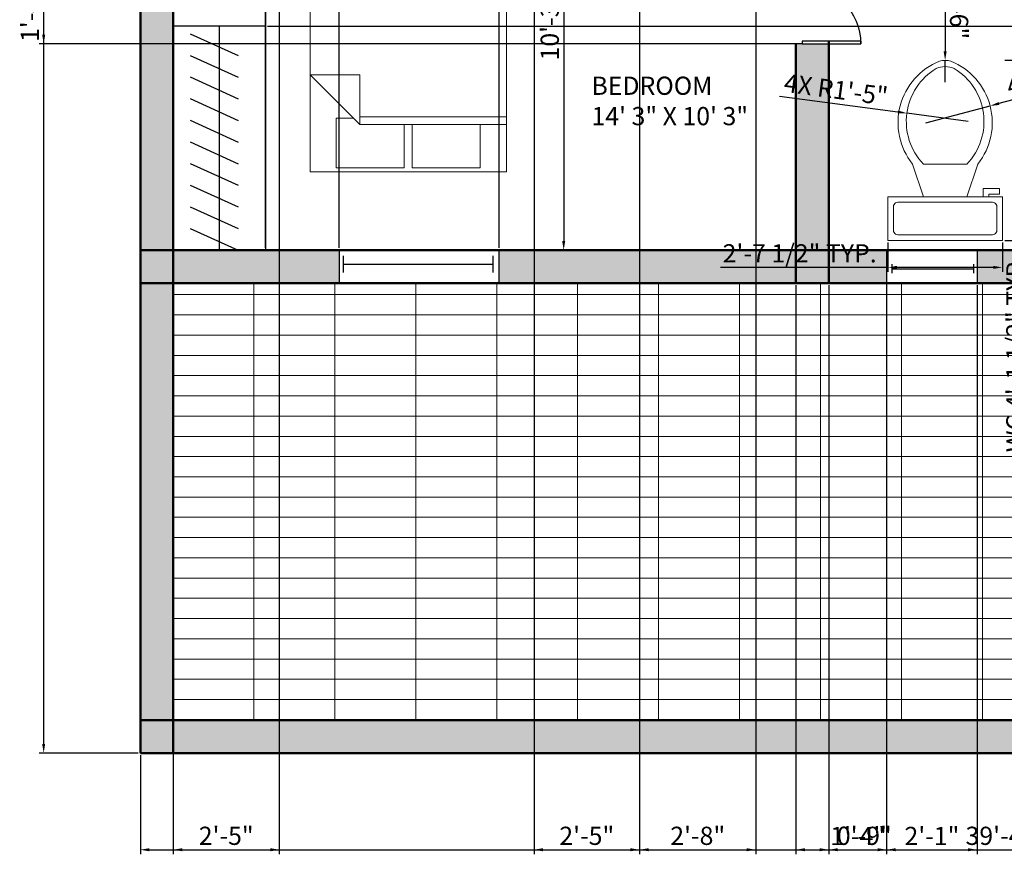
# Model space of a CAD drawing. Units: millimetres. Extents: x 2976 to 3516, y 849 to 1445.
# Tile 1 of 7: x 2981 to 3251, y 852 to 1081. Entities that reach past the tile are written whole.
import ezdxf

# ---------------------------------------------------------------- set-up
doc = ezdxf.new("R2010")
doc.units = ezdxf.units.MM
for name, color, linetype, lineweight in [('A-AREA-IDEN', 150, 'Continuous', 25), ('A-FLOR-CASE', 130, 'Continuous', 25), ('A-FLOR-FIXT', 130, 'Continuous', 18), ('A-FLOR-PATT', 3, 'Continuous', 13), ('A-WALL-PATT', 3, 'Continuous', 13), ('dimensions', 50, 'Continuous', 18), ('doors', 190, 'Continuous', 25), ('furniture', 130, 'Continuous', 18), ('walls', 80, 'Continuous', 50), ('windows', 10, 'Continuous', 25)]:
    doc.layers.add(name, color=color, linetype=linetype, lineweight=lineweight)
doc.styles.get("Standard").update_dxf_attribs({"font": 'arial.ttf'})
doc.dimstyles.new('ISO-25', dxfattribs={"dimtxt": 5, "dimasz": 2.5, "dimexe": 1.25, "dimexo": 0.625, "dimtad": 1, "dimdec": 0, "dimlunit": 3, "dimtxsty": 'Standard', "dimcen": 2.5, "dimadec": 0, "dimazin": 0, "dimtfac": 1, "dimtdec": 0, "dimtmove": 0, "dimatfit": 3, "dimfxl": 1, "dimarcsym": 0})

# ---------------------------------------------------------------- blocks, each defined once
blk = doc.blocks.new('*U2')
for p, q in [((0, 0), (0, -6)), ((40, 0), (40, -6))]:
    blk.add_line(p, q)
blk.add_lwpolyline([(0, 0), (0, 40), (1.75, 40), (1.75, 0)], close=True)
blk.add_arc((0, 0), 40, 0, 90)
blk = doc.blocks.new('*U4')
for p, q in [((0, 4), (0, 0)), ((36, 4), (36, 0)), ((0, 2), (36, 2))]:
    blk.add_line(p, q)
blk = doc.blocks.new('*U5')
for p, q in [((0, 4), (0, 0)), ((0, 2), (36, 2)), ((36, 4), (36, 0))]:
    blk.add_line(p, q)
blk = doc.blocks.new('Bed - Queen')
for p, q in [((0, -80.00003), (0, 0)), ((0, 0), (59.99999, 0)), ((59.99999, 0), (59.99999, -80.00003)), ((7.99999, -1.2), (28.79998, -1.2)), ((7.99999, -14.4), (7.99999, -1.2)), ((28.79998, -1.2), (28.79998, -14.4)), ((31.19999, -1.2), (51.99999, -1.2)), ((31.19999, -14.4), (31.19999, -1.2)), ((51.99999, -1.2), (51.99999, -16.4)), ((0, -14.4), (44.8, -14.4)), ((59.99999, -29.6), (44.8, -14.4)), ((44.8, -14.4), (44.8, -29.6)), ((44.8, -16.8), (0, -16.8)), ((51.99999, -16.4), (46.79936, -16.4)), ((44.8, -29.6), (59.99999, -29.6)), ((59.99999, -80.00003), (0, -80.00003))]:
    blk.add_line(p, q)
blk = doc.blocks.new('Toilet - top')
for p, q in [((9.5, -6), (9.5, -2)), ((-10, -8.5), (-8, -8.5)), ((-10, -9.5), (-10, -8.5)), ((-8, -8.5), (-8, -8)), ((-7, -8), (-7, -9.5)), ((-4, -8), (-6, -14)), ((4, -8), (6, -14)), ((-7, -9.5), (-10, -9.5)), ((4, -14), (-4, -14))]:
    blk.add_line(p, q)
blk.add_lwpolyline([(10.5, -8), (10.5, 0), (-10.5, 0), (-10.5, -8)], close=True)
for points in [[(8.5, -1), (-8.5, -1)], [(-9.5, -2), (-9.5, -6)], [(-8.5, -7), (8.5, -7)]]:
    blk.add_lwpolyline(points)
for centre, radius, start, end in [((-8.62, -1.88), 0.884, 81.8699, 188.1301), ((8.62, -1.88), 0.884, 351.8699, 98.1301), ((-8.62, -6.12), 0.884, 171.8699, 278.1301), ((8.62, -6.12), 0.884, 261.8699, 8.1301), ((3.52, -21.58), 12.17, 141.4691, 247.9714), ((4.2, -21.82), 11.33, 136.3677, 238.9468), ((-3.52, -21.58), 12.17, 292.0284, 38.5307), ((-4.2, -21.82), 11.33, 301.053, 43.6321), ((0, -27.88), 4, 245.7318, 294.2682), ((0, -29), 4, 254.8605, 285.1395)]:
    blk.add_arc(centre, radius, start, end)
blk = doc.blocks.new('*D16')
at = {"layer": 'Defpoints', "color": 0, "transparency": 16777216}
for p in [(3129.91, 1140.88), (3129.91, 1017.88), (3129.91, 1017.88)]:
    blk.add_point(p, dxfattribs=at)
at = {"layer": 'dimensions', "color": 0, "lineweight": -2, "transparency": 16777216}
for p, q in [((3130.53, 1140.88), (3131.16, 1140.88)), ((3129.91, 1138.38), (3129.91, 1020.38)), ((3130.53, 1017.88), (3131.16, 1017.88))]:
    blk.add_line(p, q, dxfattribs=at)
at = {"layer": 'dimensions', "color": 0, "transparency": 16777216}
for points in [[(3129.49, 1138.38), (3130.32, 1138.38), (3129.91, 1140.88)], [(3129.49, 1020.38), (3130.32, 1020.38), (3129.91, 1017.88)]]:
    blk.add_solid(points, dxfattribs=at)
at = {"layer": 'dimensions', "color": 0, "transparency": 16777216, "insert": (3126.73, 1079.38), "char_height": 5, "attachment_point": 5, "rotation": 90}
blk.add_mtext('10\'-3"', dxfattribs=at)
blk = doc.blocks.new('*D32')
at = {"layer": 'Defpoints', "color": 0, "transparency": 16777216}
for p in [(3250.35, 1070.03), (3250.35, 1020.59), (3257.77, 1020.59)]:
    blk.add_point(p, dxfattribs=at)
at = {"layer": 'dimensions', "color": 0, "lineweight": -2, "transparency": 16777216}
for p, q in [((3250.98, 1070.03), (3259.02, 1070.03)), ((3257.77, 1067.53), (3257.77, 1023.09)), ((3250.98, 1020.59), (3259.02, 1020.59)), ((3257.77, 1020.59), (3257.77, 960.93))]:
    blk.add_line(p, q, dxfattribs=at)
at = {"layer": 'dimensions', "color": 0, "transparency": 16777216}
for points in [[(3257.35, 1067.53), (3258.18, 1067.53), (3257.77, 1070.03)], [(3257.35, 1023.09), (3258.18, 1023.09), (3257.77, 1020.59)]]:
    blk.add_solid(points, dxfattribs=at)
at = {"layer": 'dimensions', "color": 0, "transparency": 16777216, "insert": (3254.56, 989.51), "char_height": 5, "attachment_point": 5, "rotation": 90}
blk.add_mtext('WC 4\'-1 1/2" TYP.', dxfattribs=at)
blk = doc.blocks.new('*D33')
at = {"layer": 'Defpoints', "color": 0, "transparency": 16777216}
for p in [(3218.93, 1020.59), (3250.35, 1020.59), (3218.93, 1013.17)]:
    blk.add_point(p, dxfattribs=at)
at = {"layer": 'dimensions', "color": 0, "lineweight": -2, "transparency": 16777216}
for p, q in [((3218.93, 1019.97), (3218.93, 1011.92)), ((3250.35, 1019.97), (3250.35, 1011.92)), ((3218.93, 1013.17), (3172.97, 1013.17)), ((3247.85, 1013.17), (3221.43, 1013.17))]:
    blk.add_line(p, q, dxfattribs=at)
at = {"layer": 'dimensions', "color": 0, "transparency": 16777216}
for points in [[(3221.43, 1013.59), (3221.43, 1012.76), (3218.93, 1013.17)], [(3247.85, 1013.59), (3247.85, 1012.76), (3250.35, 1013.17)]]:
    blk.add_solid(points, dxfattribs=at)
at = {"layer": 'dimensions', "color": 0, "transparency": 16777216, "insert": (3194.7, 1016.38), "char_height": 5, "attachment_point": 5}
blk.add_mtext('2\'-7 1/2" TYP.', dxfattribs=at)
blk = doc.blocks.new('*D38')
at = {"layer": 'Defpoints', "color": 0, "transparency": 16777216}
for p in [(3013.67, 879.88), (3485.67, 879.88), (3485.67, 853.34)]:
    blk.add_point(p, dxfattribs=at)
at = {"layer": 'dimensions', "color": 0, "lineweight": -2, "transparency": 16777216}
for p, q in [((3013.67, 879.26), (3013.67, 852.09)), ((3485.67, 879.26), (3485.67, 852.09)), ((3016.17, 853.34), (3483.17, 853.34))]:
    blk.add_line(p, q, dxfattribs=at)
at = {"layer": 'dimensions', "color": 0, "transparency": 16777216}
for points in [[(3016.17, 853.76), (3016.17, 852.92), (3013.67, 853.34)], [(3483.17, 853.76), (3483.17, 852.92), (3485.67, 853.34)]]:
    blk.add_solid(points, dxfattribs=at)
at = {"layer": 'dimensions', "color": 0, "transparency": 16777216, "insert": (3249.67, 856.52), "char_height": 5, "attachment_point": 5}
blk.add_mtext('39\'-4"', dxfattribs=at)
blk = doc.blocks.new('*D39')
at = {"layer": 'Defpoints', "color": 0, "transparency": 16777216}
for p in [(2987.13, 1407.88), (3013.67, 1407.88), (3013.67, 879.88)]:
    blk.add_point(p, dxfattribs=at)
at = {"layer": 'dimensions', "color": 0, "lineweight": -2, "transparency": 16777216}
for p, q in [((3013.05, 1407.88), (2985.88, 1407.88)), ((2987.13, 882.38), (2987.13, 1405.38)), ((3013.05, 879.88), (2985.88, 879.88))]:
    blk.add_line(p, q, dxfattribs=at)
at = {"layer": 'dimensions', "color": 0, "transparency": 16777216}
for points in [[(2986.71, 1405.38), (2987.55, 1405.38), (2987.13, 1407.88)], [(2986.71, 882.38), (2987.55, 882.38), (2987.13, 879.88)]]:
    blk.add_solid(points, dxfattribs=at)
at = {"layer": 'dimensions', "color": 0, "transparency": 16777216, "insert": (2983.95, 1143.88), "char_height": 5, "attachment_point": 5, "rotation": 90}
blk.add_mtext('44\'-0"', dxfattribs=at)
blk = doc.blocks.new('*D41')
at = {"layer": 'Defpoints', "color": 0, "transparency": 16777216}
for p in [(3022.67, 1008.88), (3512.21, 1008.88), (3013.67, 888.88)]:
    blk.add_point(p, dxfattribs=at)
at = {"layer": 'dimensions', "color": 0, "lineweight": -2, "transparency": 16777216}
for p, q in [((3023.3, 1008.88), (3513.46, 1008.88)), ((3512.21, 891.38), (3512.21, 1006.38)), ((3014.3, 888.88), (3513.46, 888.88))]:
    blk.add_line(p, q, dxfattribs=at)
at = {"layer": 'dimensions', "color": 0, "transparency": 16777216}
for points in [[(3511.79, 1006.38), (3512.63, 1006.38), (3512.21, 1008.88)], [(3511.79, 891.38), (3512.63, 891.38), (3512.21, 888.88)]]:
    blk.add_solid(points, dxfattribs=at)
at = {"layer": 'dimensions', "color": 0, "transparency": 16777216, "insert": (3509.03, 948.88), "char_height": 5, "attachment_point": 5, "rotation": 90}
blk.add_mtext('10\'-0"', dxfattribs=at)
blk = doc.blocks.new('*D52')
at = {"layer": 'Defpoints', "color": 0, "transparency": 16777216}
for p in [(3121.76, 1269.88), (3150.74, 1269.88), (3150.74, 853.34)]:
    blk.add_point(p, dxfattribs=at)
at = {"layer": 'dimensions', "color": 0, "lineweight": -2, "transparency": 16777216}
for p, q in [((3121.76, 1269.26), (3121.76, 852.09)), ((3150.74, 1269.26), (3150.74, 852.09)), ((3124.26, 853.34), (3148.24, 853.34))]:
    blk.add_line(p, q, dxfattribs=at)
at = {"layer": 'dimensions', "color": 0, "transparency": 16777216}
for points in [[(3124.26, 853.76), (3124.26, 852.92), (3121.76, 853.34)], [(3148.24, 853.76), (3148.24, 852.92), (3150.74, 853.34)]]:
    blk.add_solid(points, dxfattribs=at)
at = {"layer": 'dimensions', "color": 0, "transparency": 16777216, "insert": (3136.25, 856.52), "char_height": 5, "attachment_point": 5}
blk.add_mtext('2\'-5"', dxfattribs=at)
blk = doc.blocks.new('*D53')
at = {"layer": 'Defpoints', "color": 0, "transparency": 16777216}
for p in [(2987.13, 1090.58), (3193.67, 1090.58), (3193.67, 1074.53)]:
    blk.add_point(p, dxfattribs=at)
at = {"layer": 'dimensions', "color": 0, "lineweight": -2, "transparency": 16777216}
for p, q in [((3193.05, 1090.58), (2985.88, 1090.58)), ((2987.13, 1077.03), (2987.13, 1088.08)), ((3193.05, 1074.53), (2985.88, 1074.53))]:
    blk.add_line(p, q, dxfattribs=at)
at = {"layer": 'dimensions', "color": 0, "transparency": 16777216}
for points in [[(2986.71, 1088.08), (2987.55, 1088.08), (2987.13, 1090.58)], [(2986.71, 1077.03), (2987.55, 1077.03), (2987.13, 1074.53)]]:
    blk.add_solid(points, dxfattribs=at)
at = {"layer": 'dimensions', "color": 0, "transparency": 16777216, "insert": (2984, 1082.56), "char_height": 5, "attachment_point": 5, "rotation": 90}
blk.add_mtext('1\'-4"', dxfattribs=at)
blk = doc.blocks.new('*D57')
at = {"layer": 'Defpoints', "color": 0, "transparency": 16777216}
for p in [(3112.23, 1434.42), (3068.25, 1017.88), (3112.23, 1017.88)]:
    blk.add_point(p, dxfattribs=at)
at = {"layer": 'dimensions', "color": 0, "lineweight": -2, "transparency": 16777216}
for p, q in [((3068.25, 1018.51), (3068.25, 1435.67)), ((3112.23, 1018.51), (3112.23, 1435.67)), ((3070.75, 1434.42), (3109.73, 1434.42))]:
    blk.add_line(p, q, dxfattribs=at)
at = {"layer": 'dimensions', "color": 0, "transparency": 16777216}
for points in [[(3070.75, 1434.84), (3070.75, 1434), (3068.25, 1434.42)], [(3109.73, 1434.84), (3109.73, 1434), (3112.23, 1434.42)]]:
    blk.add_solid(points, dxfattribs=at)
at = {"layer": 'dimensions', "color": 0, "transparency": 16777216, "insert": (3090.24, 1437.6), "char_height": 5, "attachment_point": 5}
blk.add_mtext('3\'-8"', dxfattribs=at)
blk = doc.blocks.new('*D58')
at = {"layer": 'Defpoints', "color": 0, "transparency": 16777216}
for p in [(3218.58, 1008.88), (3243.44, 1008.88), (3243.44, 853.34)]:
    blk.add_point(p, dxfattribs=at)
at = {"layer": 'dimensions', "color": 0, "lineweight": -2, "transparency": 16777216}
for p, q in [((3218.58, 1008.26), (3218.58, 852.09)), ((3243.44, 1008.26), (3243.44, 852.09)), ((3221.08, 853.34), (3240.94, 853.34))]:
    blk.add_line(p, q, dxfattribs=at)
at = {"layer": 'dimensions', "color": 0, "transparency": 16777216}
for points in [[(3221.08, 853.76), (3221.08, 852.92), (3218.58, 853.34)], [(3240.94, 853.76), (3240.94, 852.92), (3243.44, 853.34)]]:
    blk.add_solid(points, dxfattribs=at)
at = {"layer": 'dimensions', "color": 0, "transparency": 16777216, "insert": (3231.01, 856.48), "char_height": 5, "attachment_point": 5}
blk.add_mtext('2\'-1"', dxfattribs=at)
blk = doc.blocks.new('*D60')
at = {"layer": 'Defpoints', "color": 0, "transparency": 16777216}
for p in [(3193.67, 1008.88), (3202.67, 1008.88), (3202.67, 853.34)]:
    blk.add_point(p, dxfattribs=at)
at = {"layer": 'dimensions', "color": 0, "lineweight": -2, "transparency": 16777216}
for p, q in [((3193.67, 1008.26), (3193.67, 852.09)), ((3202.67, 1008.26), (3202.67, 852.09)), ((3196.17, 853.34), (3200.17, 853.34)), ((3202.67, 853.34), (3219.71, 853.34))]:
    blk.add_line(p, q, dxfattribs=at)
at = {"layer": 'dimensions', "color": 0, "transparency": 16777216}
for points in [[(3196.17, 853.76), (3196.17, 852.92), (3193.67, 853.34)], [(3200.17, 853.76), (3200.17, 852.92), (3202.67, 853.34)]]:
    blk.add_solid(points, dxfattribs=at)
at = {"layer": 'dimensions', "color": 0, "transparency": 16777216, "insert": (3212.44, 856.52), "char_height": 5, "attachment_point": 5}
blk.add_mtext('0\'-9"', dxfattribs=at)
blk = doc.blocks.new('*D70')
at = {"layer": 'Defpoints', "color": 0, "transparency": 16777216}
for p in [(3218.58, 1017.88), (3202.67, 1008.88), (3218.58, 853.34)]:
    blk.add_point(p, dxfattribs=at)
at = {"layer": 'dimensions', "color": 0, "lineweight": -2, "transparency": 16777216}
for p, q in [((3218.58, 1017.26), (3218.58, 852.09)), ((3202.67, 1008.26), (3202.67, 852.09)), ((3205.17, 853.34), (3216.08, 853.34))]:
    blk.add_line(p, q, dxfattribs=at)
at = {"layer": 'dimensions', "color": 0, "transparency": 16777216}
for points in [[(3205.17, 853.76), (3205.17, 852.92), (3202.67, 853.34)], [(3216.08, 853.76), (3216.08, 852.92), (3218.58, 853.34)]]:
    blk.add_solid(points, dxfattribs=at)
at = {"layer": 'dimensions', "color": 0, "transparency": 16777216, "insert": (3210.63, 856.48), "char_height": 5, "attachment_point": 5}
blk.add_mtext('1\'-4"', dxfattribs=at)
blk = doc.blocks.new('*D72')
at = {"layer": 'Defpoints', "color": 0, "transparency": 16777216}
for p in [(3150.74, 1269.88), (3182.67, 1269.88), (3182.67, 853.34)]:
    blk.add_point(p, dxfattribs=at)
at = {"layer": 'dimensions', "color": 0, "lineweight": -2, "transparency": 16777216}
for p, q in [((3150.74, 1269.26), (3150.74, 852.09)), ((3182.67, 1269.26), (3182.67, 852.09)), ((3153.24, 853.34), (3180.17, 853.34))]:
    blk.add_line(p, q, dxfattribs=at)
at = {"layer": 'dimensions', "color": 0, "transparency": 16777216}
for points in [[(3153.24, 853.76), (3153.24, 852.92), (3150.74, 853.34)], [(3180.17, 853.76), (3180.17, 852.92), (3182.67, 853.34)]]:
    blk.add_solid(points, dxfattribs=at)
at = {"layer": 'dimensions', "color": 0, "transparency": 16777216, "insert": (3166.71, 856.52), "char_height": 5, "attachment_point": 5}
blk.add_mtext('2\'-8"', dxfattribs=at)
blk = doc.blocks.new('*D75')
at = {"layer": 'Defpoints', "color": 0, "transparency": 16777216}
for p in [(3022.67, 1338.88), (3051.83, 1338.88), (3051.83, 853.34)]:
    blk.add_point(p, dxfattribs=at)
at = {"layer": 'dimensions', "color": 0, "lineweight": -2, "transparency": 16777216}
for p, q in [((3022.67, 1338.26), (3022.67, 852.09)), ((3051.83, 1338.26), (3051.83, 852.09)), ((3025.17, 853.34), (3049.33, 853.34))]:
    blk.add_line(p, q, dxfattribs=at)
at = {"layer": 'dimensions', "color": 0, "transparency": 16777216}
for points in [[(3025.17, 853.76), (3025.17, 852.92), (3022.67, 853.34)], [(3049.33, 853.76), (3049.33, 852.92), (3051.83, 853.34)]]:
    blk.add_solid(points, dxfattribs=at)
at = {"layer": 'dimensions', "color": 0, "transparency": 16777216, "insert": (3037.25, 856.52), "char_height": 5, "attachment_point": 5}
blk.add_mtext('2\'-5"', dxfattribs=at)
blk = doc.blocks.new('*D77')
at = {"layer": 'Defpoints', "color": 0, "transparency": 16777216}
for p in [(3048, 1434.42), (3022.67, 1079.38), (3048, 1079.38)]:
    blk.add_point(p, dxfattribs=at)
at = {"layer": 'dimensions', "color": 0, "lineweight": -2, "transparency": 16777216}
for p, q in [((3022.67, 1080.01), (3022.67, 1435.67)), ((3048, 1080.01), (3048, 1435.67)), ((3025.17, 1434.42), (3045.5, 1434.42)), ((3048, 1434.42), (3076.78, 1434.42))]:
    blk.add_line(p, q, dxfattribs=at)
at = {"layer": 'dimensions', "color": 0, "transparency": 16777216}
for points in [[(3025.17, 1434.84), (3025.17, 1434), (3022.67, 1434.42)], [(3045.5, 1434.84), (3045.5, 1434), (3048, 1434.42)]]:
    blk.add_solid(points, dxfattribs=at)
at = {"layer": 'dimensions', "color": 0, "transparency": 16777216, "insert": (3063.64, 1437.63), "char_height": 5, "attachment_point": 5}
blk.add_mtext('2\'-1 1/2"', dxfattribs=at)
blk = doc.blocks.new('*D78')
at = {"layer": 'Defpoints', "color": 0, "transparency": 16777216}
for p in [(3048, 1079.38), (3512.21, 1079.38), (3048, 1017.88)]:
    blk.add_point(p, dxfattribs=at)
at = {"layer": 'dimensions', "color": 0, "lineweight": -2, "transparency": 16777216}
for p, q in [((3048.62, 1079.38), (3513.46, 1079.38)), ((3512.21, 1020.38), (3512.21, 1076.88)), ((3048.62, 1017.88), (3513.46, 1017.88))]:
    blk.add_line(p, q, dxfattribs=at)
at = {"layer": 'dimensions', "color": 0, "transparency": 16777216}
for points in [[(3511.79, 1076.88), (3512.63, 1076.88), (3512.21, 1079.38)], [(3511.79, 1020.38), (3512.63, 1020.38), (3512.21, 1017.88)]]:
    blk.add_solid(points, dxfattribs=at)
at = {"layer": 'dimensions', "color": 0, "transparency": 16777216, "insert": (3509, 1048.63), "char_height": 5, "attachment_point": 5, "rotation": 90}
blk.add_mtext('5\'-1 1/2"', dxfattribs=at)
blk = doc.blocks.new('*D79')
at = {"layer": 'Defpoints', "color": 0, "transparency": 16777216}
for p in [(3068.25, 1434.42), (3048, 1017.88), (3068.25, 1017.88)]:
    blk.add_point(p, dxfattribs=at)
at = {"layer": 'dimensions', "color": 0, "lineweight": -2, "transparency": 16777216}
for p, q in [((3048, 1018.51), (3048, 1435.67)), ((3068.25, 1018.51), (3068.25, 1435.67)), ((3050.5, 1434.42), (3065.75, 1434.42))]:
    blk.add_line(p, q, dxfattribs=at)
at = {"layer": 'dimensions', "color": 0, "transparency": 16777216}
for points in [[(3050.5, 1434.84), (3050.5, 1434), (3048, 1434.42)], [(3065.75, 1434.84), (3065.75, 1434), (3068.25, 1434.42)]]:
    blk.add_solid(points, dxfattribs=at)
at = {"layer": 'dimensions', "color": 0, "transparency": 16777216, "insert": (3058.12, 1437.6), "char_height": 5, "attachment_point": 5}
blk.add_mtext('1\'-8"', dxfattribs=at)
blk = doc.blocks.new('*D86')
at = {"layer": 'Defpoints', "color": 0, "transparency": 16777216}
for p in [(3246.98, 1057.5), (3229.38, 1052.88)]:
    blk.add_point(p, dxfattribs=at)
at = {"layer": 'dimensions', "color": 0, "lineweight": -2, "transparency": 16777216}
for p, q in [((3281.1, 1066.47), (3249.4, 1058.14)), ((3229.38, 1052.88), (3246.98, 1057.5))]:
    blk.add_line(p, q, dxfattribs=at)
at = {"layer": 'dimensions', "color": 0, "transparency": 16777216}
blk.add_solid([(3249.3, 1058.54), (3249.51, 1057.74), (3246.98, 1057.5)], dxfattribs=at)
at = {"layer": 'dimensions', "color": 0, "transparency": 16777216, "insert": (3265.65, 1065.69), "char_height": 5, "attachment_point": 5, "rotation": 14.7202}
blk.add_mtext('4X R1\'-6"', dxfattribs=at)
blk = doc.blocks.new('*D87')
at = {"layer": 'Defpoints', "color": 0, "transparency": 16777216}
for p in [(3224.13, 1055.49), (3240.93, 1053.23)]:
    blk.add_point(p, dxfattribs=at)
at = {"layer": 'dimensions', "color": 0, "lineweight": -2, "transparency": 16777216}
for p, q in [((3189.17, 1060.19), (3221.65, 1055.83)), ((3240.93, 1053.23), (3224.13, 1055.49))]:
    blk.add_line(p, q, dxfattribs=at)
at = {"layer": 'dimensions', "color": 0, "transparency": 16777216}
blk.add_solid([(3221.7, 1056.24), (3221.59, 1055.41), (3224.13, 1055.49)], dxfattribs=at)
at = {"layer": 'dimensions', "color": 0, "transparency": 16777216, "insert": (3204.59, 1061.32), "char_height": 5, "attachment_point": 5, "rotation": 352.3418}
blk.add_mtext('4X R1\'-5"', dxfattribs=at)
blk = doc.blocks.new('*D88')
at = {"layer": 'Defpoints', "color": 0, "transparency": 16777216}
for p in [(3234.64, 1069.96), (3234.64, 1063.98)]:
    blk.add_point(p, dxfattribs=at)
at = {"layer": 'dimensions', "color": 0, "lineweight": -2, "transparency": 16777216}
for p, q in [((3234.64, 1105.24), (3234.64, 1072.46)), ((3234.64, 1063.98), (3234.64, 1069.96))]:
    blk.add_line(p, q, dxfattribs=at)
at = {"layer": 'dimensions', "color": 0, "transparency": 16777216}
blk.add_solid([(3235.06, 1072.46), (3234.22, 1072.46), (3234.64, 1069.96)], dxfattribs=at)
at = {"layer": 'dimensions', "color": 0, "transparency": 16777216, "insert": (3237.82, 1090.1), "char_height": 5, "attachment_point": 5, "rotation": 270.0033}
blk.add_mtext('4X R0\'-6"', dxfattribs=at)

msp = doc.modelspace()

# ---------------------------------------------------------------- hatches: boundary and pattern name
at = {"layer": 'A-FLOR-PATT'}
h = msp.add_hatch(dxfattribs=at)
h.set_pattern_fill('GRATE', color=256, scale=7)
h.paths.add_polyline_path([(3383.67, 1008.88), (3022.67, 1008.88), (3022.67, 888.88), (3383.67, 888.88)])
at = {"layer": 'A-WALL-PATT'}
h = msp.add_hatch(color=256, dxfattribs=at)
h.dxf.hatch_style = 1
h.paths.add_polyline_path([(3022.67, 1398.88), (3013.67, 1398.88), (3013.67, 1278.88), (3022.67, 1278.88)])
h.paths.add_polyline_path([(3082.67, 1278.88), (3022.67, 1278.88), (3022.67, 1269.88), (3082.67, 1269.88)])
h.paths.add_polyline_path([(3022.67, 1278.88), (3013.67, 1278.88), (3013.67, 1269.88), (3022.67, 1269.88)])
h.paths.add_polyline_path([(3091.67, 1278.88), (3082.67, 1278.88), (3082.67, 1269.88), (3091.67, 1269.88)])
h.paths.add_polyline_path([(3121.76, 1278.88), (3091.67, 1278.88), (3091.67, 1269.88), (3121.76, 1269.88), (3121.76, 1272.56)])
h.paths.add_polyline_path([(3022.67, 1269.88), (3013.67, 1269.88), (3013.67, 1149.88), (3022.67, 1149.88)])
h.paths.add_polyline_path([(3022.67, 1140.88), (3013.67, 1140.88), (3013.67, 1017.88), (3022.67, 1017.88)])
h.paths.add_polyline_path([(3022.67, 1149.88), (3013.67, 1149.88), (3013.67, 1140.88), (3022.67, 1140.88)])
h.paths.add_polyline_path([(3082.67, 1149.88), (3022.67, 1149.88), (3022.67, 1140.88), (3082.67, 1140.88)])
h.paths.add_polyline_path([(3091.67, 1149.88), (3082.67, 1149.88), (3082.67, 1140.88), (3091.67, 1140.88)])
h.paths.add_polyline_path([(3143.42, 1147.68), (3143.42, 1149.88), (3091.67, 1149.88), (3091.67, 1140.88), (3144.23, 1140.88, -0.059251)])
h.paths.add_polyline_path([(3193.67, 1149.88), (3172.4, 1149.88), (3172.4, 1147.68), (3172.4, 1140.88), (3193.67, 1140.88)])
h.paths.add_polyline_path([(3202.67, 1149.88), (3193.67, 1149.88), (3193.67, 1140.88), (3202.67, 1140.88)])
h.paths.add_polyline_path([(3272.67, 1149.88), (3262.67, 1149.88), (3262.67, 1140.88), (3272.67, 1140.88)])
h.paths.add_polyline_path([(3272.67, 1140.88), (3262.67, 1140.88), (3262.67, 1083.88), (3272.67, 1083.88)])
h.paths.add_polyline_path([(3202.67, 1140.88), (3193.67, 1140.88), (3193.67, 1090.58), (3195.4, 1090.58, -0.118064), (3202.67, 1088.84)])
h.paths.add_polyline_path([(3202.67, 1074.53), (3195.4, 1074.53), (3193.67, 1074.53), (3193.67, 1017.88), (3202.67, 1017.88)])
h.paths.add_polyline_path([(3202.67, 1017.88), (3193.67, 1017.88), (3193.67, 1008.88), (3202.67, 1008.88)])
h.paths.add_polyline_path([(3193.67, 1017.88), (3112.23, 1017.88), (3112.23, 1008.88), (3193.67, 1008.88)])
h.paths.add_polyline_path([(3068.25, 1017.88), (3022.67, 1017.88), (3022.67, 1008.88), (3068.25, 1008.88)])
h.paths.add_polyline_path([(3022.67, 1017.88), (3013.67, 1017.88), (3013.67, 1008.88), (3022.67, 1008.88)])
h.paths.add_polyline_path([(3272.67, 1074.88), (3262.67, 1074.88), (3262.67, 1017.88), (3271.67, 1017.88), (3272.67, 1017.88)])
h.paths.add_polyline_path([(3272.67, 1083.88), (3262.67, 1083.88), (3262.67, 1074.88), (3272.67, 1074.88)])
h.paths.add_polyline_path([(3284.41, 1082.91), (3284.41, 1083.88), (3272.67, 1083.88), (3272.67, 1074.88), (3284.41, 1074.88)])
h.paths.add_polyline_path([(3383.67, 1083.88), (3300.46, 1083.88), (3300.46, 1082.91, -0.131652), (3298.31, 1074.88), (3383.67, 1074.88)])
h.paths.add_polyline_path([(3392.67, 1083.88), (3383.67, 1083.88), (3383.67, 1074.88), (3392.67, 1074.88)])
h.paths.add_polyline_path([(3392.67, 1074.88), (3383.67, 1074.88), (3383.67, 1017.88), (3392.67, 1017.88)])
h.paths.add_polyline_path([(3392.67, 1017.88), (3383.67, 1017.88), (3383.67, 1008.88), (3392.67, 1008.88)])
h.paths.add_polyline_path([(3383.67, 1017.88), (3347.17, 1017.88), (3347.17, 1008.88), (3383.67, 1008.88)])
h.paths.add_polyline_path([(3303.78, 1017.88), (3272.67, 1017.88), (3272.67, 1008.88), (3303.78, 1008.88)])
h.paths.add_polyline_path([(3272.67, 1017.88), (3271.67, 1017.88), (3262.67, 1017.88), (3262.67, 1008.88), (3272.67, 1008.88)])
h.paths.add_polyline_path([(3262.67, 1017.88), (3243.44, 1017.88), (3243.44, 1008.88), (3262.67, 1008.88)])
h.paths.add_polyline_path([(3218.58, 1017.88), (3202.67, 1017.88), (3202.67, 1008.88), (3218.58, 1008.88)])
h.paths.add_polyline_path([(3392.67, 1209.88), (3383.67, 1209.88), (3383.67, 1083.88), (3392.67, 1083.88)])
h.paths.add_polyline_path([(3392.67, 1218.88), (3383.67, 1218.88), (3383.67, 1209.88), (3392.67, 1209.88)])
h.paths.add_polyline_path([(3392.67, 1246.1), (3383.67, 1246.1), (3383.67, 1218.88), (3392.67, 1218.88)])
h.paths.add_polyline_path([(3383.67, 1218.88), (3251.67, 1218.88), (3251.67, 1209.88), (3383.67, 1209.88)])
h.paths.add_polyline_path([(3251.67, 1287.88), (3242.67, 1287.88), (3242.67, 1218.88), (3251.67, 1218.88)])
h.paths.add_polyline_path([(3251.67, 1218.88), (3242.67, 1218.88), (3242.67, 1209.88), (3251.67, 1209.88)])
h.paths.add_polyline_path([(3251.67, 1398.88), (3242.67, 1398.88), (3242.67, 1296.88), (3251.67, 1296.88)])
h.paths.add_polyline_path([(3251.67, 1296.88), (3242.67, 1296.88), (3242.67, 1287.88), (3251.67, 1287.88)])
h.paths.add_polyline_path([(3242.67, 1296.88), (3182.67, 1296.88), (3182.67, 1287.88), (3242.67, 1287.88)])
h.paths.add_polyline_path([(3182.67, 1296.88), (3173.67, 1296.88), (3173.67, 1287.88), (3182.67, 1287.88)])
h.paths.add_polyline_path([(3182.67, 1287.88), (3173.67, 1287.88), (3173.67, 1278.88), (3182.67, 1278.88)])
h.paths.add_polyline_path([(3182.67, 1278.88), (3173.67, 1278.88), (3173.67, 1269.88), (3182.67, 1269.88)])
h.paths.add_polyline_path([(3173.67, 1278.88), (3150.05, 1278.88, -0.054989), (3150.74, 1272.56), (3150.74, 1269.88), (3173.67, 1269.88)])
h.paths.add_polyline_path([(3182.67, 1398.88), (3173.67, 1398.88), (3173.67, 1296.88), (3182.67, 1296.88)])
h.paths.add_polyline_path([(3182.67, 1407.88), (3173.67, 1407.88), (3173.67, 1398.88), (3182.67, 1398.88)])
h.paths.add_polyline_path([(3173.67, 1407.88), (3104.59, 1407.88), (3104.59, 1398.88), (3173.67, 1398.88)])
h.paths.add_polyline_path([(3060.33, 1407.88), (3022.67, 1407.88), (3022.67, 1398.88), (3060.33, 1398.88)])
h.paths.add_polyline_path([(3022.67, 1407.88), (3013.67, 1407.88), (3013.67, 1398.88), (3022.67, 1398.88)])
h.paths.add_polyline_path([(3196.7, 1407.88), (3182.67, 1407.88), (3182.67, 1398.88), (3196.7, 1398.88)])
h.paths.add_polyline_path([(3242.67, 1407.88), (3223.57, 1407.88), (3223.57, 1398.88), (3242.67, 1398.88)])
h.paths.add_polyline_path([(3251.67, 1407.88), (3242.67, 1407.88), (3242.67, 1398.88), (3251.67, 1398.88)])
h.paths.add_polyline_path([(3295.02, 1407.88), (3251.67, 1407.88), (3251.67, 1398.88), (3295.02, 1398.88)])
h.paths.add_polyline_path([(3383.67, 1407.88), (3338.5, 1407.88), (3338.5, 1398.88), (3383.67, 1398.88)])
h.paths.add_polyline_path([(3392.67, 1407.88), (3383.67, 1407.88), (3383.67, 1398.88), (3392.67, 1398.88)])
h.paths.add_polyline_path([(3392.67, 1398.88), (3383.67, 1398.88), (3383.67, 1273.3, -0.079613), (3392.67, 1275.07)])
h = msp.add_hatch(color=256, dxfattribs=at)
h.dxf.hatch_style = 1
h.paths.add_polyline_path([(3392.67, 1008.88), (3383.67, 1008.88), (3383.67, 888.88), (3392.67, 888.88)])
h.paths.add_polyline_path([(3392.67, 888.88), (3383.67, 888.88), (3383.67, 879.88), (3392.67, 879.88)])
h.paths.add_polyline_path([(3022.67, 1008.88), (3013.67, 1008.88), (3013.67, 888.88), (3022.67, 888.88)])
h.paths.add_polyline_path([(3022.67, 888.88), (3013.67, 888.88), (3013.67, 879.88), (3022.67, 879.88)])
h.paths.add_polyline_path([(3383.67, 888.88), (3022.67, 888.88), (3022.67, 879.88), (3383.67, 879.88)])

# ---------------------------------------------------------------- linework, layer by layer
at = {"layer": 'A-FLOR-CASE'}
for p, q in [((3048, 1079.38), (3022.67, 1079.38)), ((3035.34, 1079.38), (3035.34, 1017.88)), ((3027.38, 1077.29), (3040.55, 1071.31)), ((3027.38, 1071.36), (3040.55, 1065.37)), ((3027.38, 1065.42), (3040.55, 1059.44)), ((3027.38, 1059.48), (3040.55, 1053.5)), ((3027.38, 1053.55), (3040.55, 1047.56)), ((3027.38, 1047.61), (3040.55, 1041.63)), ((3027.38, 1041.67), (3040.55, 1035.69)), ((3027.38, 1035.74), (3040.55, 1029.75)), ((3027.38, 1029.8), (3040.55, 1023.82)), ((3027.38, 1023.86), (3040.55, 1017.88))]:
    msp.add_line(p, q, dxfattribs=at)
msp.add_lwpolyline([(3022.67, 1140.88), (3048, 1140.88), (3048, 1017.88), (3022.67, 1017.88)], close=True, dxfattribs=at)
at = {"layer": 'walls'}
for p, q in [((3013.67, 1407.88), (3013.67, 1008.88)), ((3022.67, 1407.88), (3022.67, 1008.88)), ((3193.67, 1074.53), (3193.67, 1008.88)), ((3202.67, 1075.23), (3202.67, 1008.88)), ((3013.67, 1017.88), (3271.67, 1017.88)), ((3013.67, 1008.88), (3392.67, 1008.88)), ((3013.67, 1008.88), (3013.67, 879.88)), ((3022.67, 1008.88), (3022.67, 879.88)), ((3392.67, 888.88), (3013.67, 888.88)), ((3392.67, 879.88), (3013.67, 879.88))]:
    msp.add_line(p, q, dxfattribs=at)
at = {"layer": 'windows'}
for p, q in [((3068.25, 1017.88), (3068.25, 1008.88)), ((3112.23, 1008.88), (3112.23, 1017.88)), ((3218.58, 1017.88), (3218.58, 1008.88)), ((3243.44, 1017.88), (3243.44, 1008.88))]:
    msp.add_line(p, q, dxfattribs=at)

# ---------------------------------------------------------------- block references
at = {"layer": 'A-FLOR-FIXT', "xscale": 1.496177724149161, "yscale": 1.496177724149161, "zscale": 1.496177724149161, "rotation": 180}
msp.add_blockref('Toilet - top', (3234.64, 1020.59), dxfattribs=at)
at = {"layer": 'doors', "xscale": -0.4013541687362427, "yscale": 0.4013541687362427, "zscale": 0.4013541687362427, "rotation": 270}
msp.add_blockref('*U2', (3195.4, 1074.53), dxfattribs=at)
at = {"layer": 'furniture', "xscale": 0.8990276149147879, "yscale": 0.8990276149147879, "zscale": 0.8990276149147879, "rotation": 180}
msp.add_blockref('Bed - Queen', (3114.2, 1039.41), dxfattribs=at)
at = {"layer": 'windows'}
for name, p, xscale, yscale, zscale in [('*U4', (3069.37, 1011.76), 1.141608635997284, 1.141608635997284, 1.141608635997284), ('*U5', (3219.96, 1011.55), 0.6246542558083853, 0.6246542558083853, 0.6246542558083853)]:
    msp.add_blockref(name, p, dxfattribs=dict(at, xscale=xscale, yscale=yscale, zscale=zscale))

# ---------------------------------------------------------------- texts
at = {"layer": 'A-AREA-IDEN', "insert": (3137.54, 1065.52), "char_height": 5, "attachment_point": 1}
msp.add_mtext_dynamic_manual_height_columns('BEDROOM \\P14\' 3" X 10\' 3"', width=48.3635, gutter_width=12.5, heights=[0], dxfattribs=at)

# ---------------------------------------------------------------- dimensions: what is measured, and where the dimension line sits
at = {"layer": 'dimensions'}
for base, p1, p2, picture, middle in [((3048, 1434.42), (3022.67, 1079.38), (3048, 1079.38), '*D77', (3063.64, 1437.63)), ((3068.248, 1434.4215), (3047.9988, 1017.8815), (3068.248, 1017.8815), '*D79', (3058.1234, 1437.5993)), ((3112.23, 1434.42), (3068.25, 1017.88), (3112.23, 1017.88), '*D57', (3090.24, 1437.6)), ((3051.83, 853.34), (3022.67, 1338.88), (3051.83, 1338.88), '*D75', (3037.25, 856.52)), ((3150.74, 853.34), (3121.76, 1269.88), (3150.74, 1269.88), '*D52', (3136.25, 856.52)), ((3182.67, 853.34), (3150.74, 1269.88), (3182.67, 1269.88), '*D72', (3166.71, 856.52)), ((3218.58, 853.34), (3202.67, 1008.88), (3218.58, 1017.88), '*D70', (3210.63, 856.48)), ((3202.67, 853.34), (3193.67, 1008.88), (3202.67, 1008.88), '*D60', (3212.44, 856.52)), ((3243.44, 853.34), (3218.58, 1008.88), (3243.44, 1008.88), '*D58', (3231.01, 856.48)), ((3485.67, 853.34), (3013.67, 879.88), (3485.67, 879.88), '*D38', (3249.67, 856.52))]:
    dim = msp.add_linear_dim(base=base, p1=p1, p2=p2, dimstyle='ISO-25', override={"dimdec": 1, "dimlfac": 1, "dimrnd": 0, "dimzin": 1, "dimdsep": 46, "dimlunit": 4, "dimfrac": 2}, dxfattribs=at)
    dim.commit()
    dim.dimension.update_dxf_attribs({"geometry": picture, "text_midpoint": middle})
for base, p1, p2, override, picture, middle in [((2987.13, 1407.88), (3013.67, 879.88), (3013.67, 1407.88), {"dimdec": 1, "dimlfac": 1, "dimrnd": 0, "dimzin": 1, "dimdsep": 46, "dimlunit": 4, "dimfrac": 2}, '*D39', (2983.95, 1143.88)), ((3129.91, 1017.88), (3129.91, 1140.88), (3129.91, 1017.88), {"dimclrd": 0, "dimclre": 0, "dimclrt": 0}, '*D16', (3126.73, 1079.38)), ((2987.1315, 1090.5844), (3193.6715, 1074.5303), (3193.6715, 1090.5844), {"dimdec": 1, "dimlfac": 1, "dimrnd": 0, "dimzin": 1, "dimdsep": 46, "dimlunit": 4, "dimfrac": 2}, '*D53', (2983.9963, 1082.5574)), ((3512.21, 1079.38), (3048, 1017.88), (3048, 1079.38), {"dimdec": 1, "dimlfac": 1, "dimrnd": 0, "dimzin": 1, "dimdsep": 46, "dimlunit": 4, "dimfrac": 2}, '*D78', (3509, 1048.63)), ((3512.21, 1008.88), (3013.67, 888.88), (3022.67, 1008.88), {"dimdec": 1, "dimlfac": 1, "dimrnd": 0, "dimzin": 1, "dimdsep": 46, "dimlunit": 4, "dimfrac": 2}, '*D41', (3509.03, 948.88))]:
    dim = msp.add_linear_dim(base=base, p1=p1, p2=p2, angle=90, dimstyle='ISO-25', override=override, dxfattribs=at)
    dim.commit()
    dim.dimension.update_dxf_attribs({"geometry": picture, "text_midpoint": middle})
for center, mpoint, picture, middle in [((3234.64, 1063.98), (3234.64, 1069.96), '*D88', (3237.82, 1090.1)), ((3229.38, 1052.88), (3246.98, 1057.5), '*D86', (3265.65, 1065.69)), ((3240.93, 1053.23), (3224.13, 1055.49), '*D87', (3204.59, 1061.32))]:
    dim = msp.add_radius_dim(center=center, mpoint=mpoint, text='4X <>', dimstyle='ISO-25', override={"dimdec": 1, "dimlfac": 1, "dimrnd": 0, "dimzin": 1, "dimdsep": 46, "dimlunit": 4, "dimfrac": 2}, dxfattribs=at)
    dim.commit()
    dim.dimension.update_dxf_attribs({"geometry": picture, "text_midpoint": middle})
for base, p1, p2, angle, text, picture, middle in [((3257.77, 1020.59), (3250.35, 1070.03), (3250.35, 1020.59), 270, 'WC <> TYP.', '*D32', (3254.56, 989.51)), ((3218.93, 1013.17), (3250.35, 1020.59), (3218.93, 1020.59), 180, '<> TYP.', '*D33', (3194.7, 1016.38))]:
    dim = msp.add_linear_dim(base=base, p1=p1, p2=p2, angle=angle, text=text, dimstyle='ISO-25', override={"dimdec": 1, "dimlfac": 1, "dimrnd": 0, "dimzin": 1, "dimdsep": 46, "dimlunit": 4, "dimfrac": 2}, dxfattribs=at)
    dim.commit()
    dim.dimension.update_dxf_attribs({"geometry": picture, "text_midpoint": middle})

doc.saveas('drawing.dxf')
